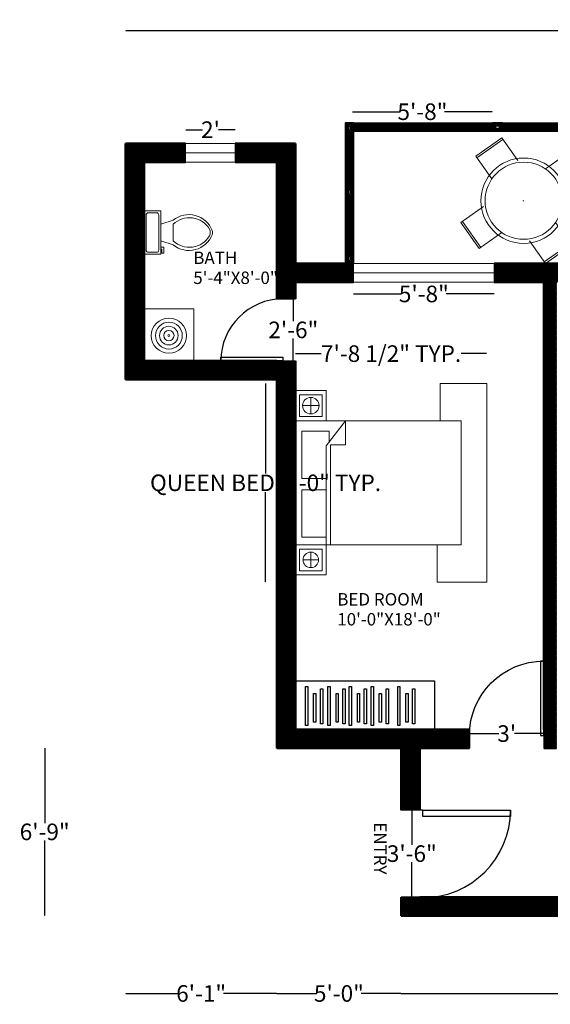
# Model space of a CAD drawing. Units: inches. Extents: x 348 to 1197, y 2602 to 3078.
# Tile 1 of 4: x 348 to 604, y 2602 to 3078. Entities that reach past the tile are written whole.
import ezdxf

# ---------------------------------------------------------------- set-up
doc = ezdxf.new("R2010")
doc.units = ezdxf.units.IN
doc.header["$MEASUREMENT"] = 0
for name, color, linetype, lineweight in [('A-ANNO-DIMS', 20, 'Continuous', 18), ('A-AREA-IDEN', 104, 'Continuous', 18), ('A-FLOR-CASE', 5, 'Continuous', 25), ('A-FLOR-FIXT', 9, 'Continuous', 18), ('A-WALL-PATT', 250, 'Continuous', 13), ('balcony', 201, 'Continuous', 25), ('bed', 5, 'Continuous', 18), ('doors', 1, 'Continuous', 25), ('table', 6, 'Continuous', 18), ('walls', 4, 'Continuous', 50), ('windows', 2, 'Continuous', 18)]:
    doc.layers.add(name, color=color, linetype=linetype, lineweight=lineweight)
doc.styles.get("Standard").update_dxf_attribs({"font": 'arial.ttf'})
doc.dimstyles.get("Standard").update_dxf_attribs({"dimtxt": 8, "dimasz": 0.18, "dimexe": 0.18, "dimexo": 0.0625, "dimgap": 0.09, "dimtad": 0, "dimtih": 1, "dimtoh": 1, "dimdec": 0, "dimzin": 0, "dimdsep": 46, "dimlunit": 3, "dimtxsty": 'Standard', "dimblk": 'DOT', "dimcen": 0.09, "dimse1": 1, "dimse2": 1, "dimadec": 0, "dimazin": 0, "dimtfac": 1, "dimtdec": 0, "dimtofl": 0, "dimtmove": 0, "dimatfit": 3, "dimfxl": 1, "dimtolj": 1, "dimtzin": 0, "dimarcsym": 0})

# ---------------------------------------------------------------- blocks, each defined once
blk = doc.blocks.new('*U8')
for p, q in [((0, 0), (0, -6)), ((24, 0), (24, -6))]:
    blk.add_line(p, q)
blk.add_lwpolyline([(0, 0), (0, 24), (1.75, 24), (1.75, 0)], close=True)
blk.add_arc((0, 0), 24, 360, 90)
blk = doc.blocks.new('*U10')
for p, q in [((0, 0), (0, -6)), ((30, 0), (30, -6))]:
    blk.add_line(p, q)
blk.add_lwpolyline([(0, 0), (0, 30), (1.75, 30), (1.75, 0)], close=True)
blk.add_arc((0, 0), 30, 0, 90)
blk = doc.blocks.new('*U9')
for p, q in [((0, 0), (0, -6)), ((36, 0), (36, -6))]:
    blk.add_line(p, q)
blk.add_lwpolyline([(0, 0), (0, 36), (1.75, 36), (1.75, 0)], close=True)
blk.add_arc((0, 0), 36, 0, 90)
blk = doc.blocks.new('*U13')
for p, q in [((5.98, 9.51), (1.98, 9.5)), ((7.99, 4.02), (13.99, 6.03)), ((13.99, 4.03), (14.01, -3.97)), ((8.01, -3.98), (14.01, -5.97)), ((8.01, -6.98), (9.51, -6.98)), ((8.52, -7.98), (8.02, -7.98)), ((8.52, -9.98), (8.52, -7.98)), ((9.51, -6.98), (9.52, -9.98)), ((9.52, -9.98), (8.52, -9.98))]:
    blk.add_line(p, q)
blk.add_lwpolyline([(7.98, 10.51), (-0.02, 10.5), (0.02, -10.5), (8.02, -10.48)], close=True)
for points in [[(0.98, 8.5), (1.02, -8.5)], [(7.02, -8.49), (6.98, 8.51)], [(2.02, -9.5), (6.02, -9.49)]]:
    blk.add_lwpolyline(points)
for centre, radius, start, end in [((6.11, 8.64), 0.884, 351.9774, 98.2376), ((1.86, 8.63), 0.884, 81.9774, 188.2376), ((21.59, -3.48), 12.17, 22.136, 128.6382), ((21.83, -4.16), 11.33, 31.1605, 133.7396), ((27.88, 0.05), 4, 335.8394, 24.3757), ((29, 0.05), 4, 344.9681, 15.247), ((21.57, 3.56), 12.17, 231.5766, 338.079), ((21.81, 4.24), 11.33, 226.4753, 329.0544), ((1.89, -8.62), 0.884, 171.9774, 278.2376), ((6.14, -8.61), 0.884, 261.9774, 8.2376)]:
    blk.add_arc(centre, radius, start, end)
blk = doc.blocks.new('*U14')
at = {"layer": 'table'}
for p, q in [((-7.7, -6.73), (-7.7, 6.73)), ((-7.7, 6.73), (7.7, 6.73)), ((-7.7, 5.73), (7.7, 5.73)), ((7.7, 6.73), (7.7, -6.73))]:
    blk.add_line(p, q, dxfattribs=at)
blk = doc.blocks.new('*U15')
at = {"layer": 'table', "transparency": 16777216}
blk.add_blockref('*U14', (596.31, 3015.18), dxfattribs=at)
for p, rotation in [((570.95, 2992.17), 90), ((619.32, 2989.82), 270), ((593.96, 2966.81), 180)]:
    blk.add_blockref('*U14', p, dxfattribs=dict(at, rotation=rotation))
blk = doc.blocks.new('_Dot')
at = {"color": 0, "linetype": 'ByBlock', "lineweight": -2}
blk.add_line((-0.5, 0), (-1, 0), dxfattribs=at)
at = {"color": 0, "linetype": 'ByBlock', "const_width": 0.5}
blk.add_lwpolyline([(-0.25, 0, 1), (0.25, 0, 1)], format="xyb", close=True, dxfattribs=at)
blk = doc.blocks.new('*D19')
at = {"layer": 'A-ANNO-DIMS', "color": 0, "lineweight": -2, "transparency": 16777216}
for p, q in [((428.5, 3024.92), (436.48, 3024.92)), ((452.14, 3024.92), (444.16, 3024.92))]:
    blk.add_line(p, q, dxfattribs=at)
at = {"layer": 'Defpoints', "color": 0, "transparency": 16777216}
for p in [(452.32, 3024.92), (428.32, 3018.2), (452.32, 3018.2)]:
    blk.add_point(p, dxfattribs=at)
at = {"layer": 'A-ANNO-DIMS', "color": 0, "lineweight": -2, "transparency": 16777216, "xscale": 0.18, "yscale": 0.18, "zscale": 0.18, "rotation": 180}
blk.add_blockref('_Dot', (428.32, 3024.92), dxfattribs=at)
at = {"layer": 'A-ANNO-DIMS', "color": 0, "lineweight": -2, "transparency": 16777216, "xscale": 0.18, "yscale": 0.18, "zscale": 0.18}
blk.add_blockref('_Dot', (452.32, 3024.92), dxfattribs=at)
at = {"layer": 'A-ANNO-DIMS', "color": 0, "transparency": 16777216, "insert": (440.32, 3024.92), "char_height": 8, "attachment_point": 5}
blk.add_mtext("\\A1;2'", dxfattribs=at)
blk = doc.blocks.new('*D20')
at = {"layer": 'A-ANNO-DIMS', "color": 0, "lineweight": -2, "transparency": 16777216}
for p, q in [((509, 3033.6), (531.92, 3033.6)), ((576.28, 3033.6), (553.36, 3033.6))]:
    blk.add_line(p, q, dxfattribs=at)
at = {"layer": 'Defpoints', "color": 0, "transparency": 16777216}
for p in [(576.46, 3033.6), (508.82, 3027.67), (576.46, 3027.67)]:
    blk.add_point(p, dxfattribs=at)
at = {"layer": 'A-ANNO-DIMS', "color": 0, "lineweight": -2, "transparency": 16777216, "xscale": 0.18, "yscale": 0.18, "zscale": 0.18, "rotation": 180}
blk.add_blockref('_Dot', (508.82, 3033.6), dxfattribs=at)
at = {"layer": 'A-ANNO-DIMS', "color": 0, "lineweight": -2, "transparency": 16777216, "xscale": 0.18, "yscale": 0.18, "zscale": 0.18}
blk.add_blockref('_Dot', (576.46, 3033.6), dxfattribs=at)
at = {"layer": 'A-ANNO-DIMS', "color": 0, "transparency": 16777216, "insert": (542.64, 3033.6), "char_height": 8, "attachment_point": 5}
blk.add_mtext('\\A1;5\'-8"', dxfattribs=at)
blk = doc.blocks.new('*D23')
at = {"layer": 'A-ANNO-DIMS', "color": 0, "lineweight": -2, "transparency": 16777216}
for p, q in [((537.51, 2696.02), (537.51, 2679.38)), ((537.51, 2654.38), (537.51, 2671.03))]:
    blk.add_line(p, q, dxfattribs=at)
at = {"layer": 'Defpoints', "color": 0, "transparency": 16777216}
for p in [(532.32, 2696.2), (532.32, 2654.2), (537.51, 2654.2)]:
    blk.add_point(p, dxfattribs=at)
at = {"layer": 'A-ANNO-DIMS', "color": 0, "lineweight": -2, "transparency": 16777216, "xscale": 0.18, "yscale": 0.18, "zscale": 0.18}
for p, rotation in [((537.51, 2696.2), 90), ((537.51, 2654.2), 270)]:
    blk.add_blockref('_Dot', p, dxfattribs=dict(at, rotation=rotation))
at = {"layer": 'A-ANNO-DIMS', "color": 0, "transparency": 16777216, "insert": (537.51, 2675.2), "char_height": 8, "attachment_point": 5}
blk.add_mtext('\\A1;3\'-6"', dxfattribs=at)
blk = doc.blocks.new('*D24')
at = {"layer": 'A-ANNO-DIMS', "color": 0, "lineweight": -2, "transparency": 16777216}
for p, q in [((565.5, 2733.19), (579.55, 2733.19)), ((601.14, 2733.19), (587.09, 2733.19))]:
    blk.add_line(p, q, dxfattribs=at)
at = {"layer": 'Defpoints', "color": 0, "transparency": 16777216}
for p in [(601.32, 2733.19), (565.32, 2726.2), (601.32, 2726.2)]:
    blk.add_point(p, dxfattribs=at)
at = {"layer": 'A-ANNO-DIMS', "color": 0, "lineweight": -2, "transparency": 16777216, "xscale": 0.18, "yscale": 0.18, "zscale": 0.18, "rotation": 180}
blk.add_blockref('_Dot', (565.32, 2733.19), dxfattribs=at)
at = {"layer": 'A-ANNO-DIMS', "color": 0, "lineweight": -2, "transparency": 16777216, "xscale": 0.18, "yscale": 0.18, "zscale": 0.18}
blk.add_blockref('_Dot', (601.32, 2733.19), dxfattribs=at)
at = {"layer": 'A-ANNO-DIMS', "color": 0, "transparency": 16777216, "insert": (583.32, 2733.19), "char_height": 8, "attachment_point": 5}
blk.add_mtext("\\A1;3'", dxfattribs=at)
blk = doc.blocks.new('*D28')
at = {"layer": 'A-ANNO-DIMS', "color": 0, "lineweight": -2, "transparency": 16777216}
for p, q in [((509.5, 2945.57), (532.59, 2945.57)), ((577.14, 2945.57), (554.04, 2945.57))]:
    blk.add_line(p, q, dxfattribs=at)
at = {"layer": 'Defpoints', "color": 0, "transparency": 16777216}
for p in [(509.32, 2951.2), (577.32, 2951.2), (577.32, 2945.57)]:
    blk.add_point(p, dxfattribs=at)
at = {"layer": 'A-ANNO-DIMS', "color": 0, "lineweight": -2, "transparency": 16777216, "xscale": 0.18, "yscale": 0.18, "zscale": 0.18, "rotation": 180}
blk.add_blockref('_Dot', (509.32, 2945.57), dxfattribs=at)
at = {"layer": 'A-ANNO-DIMS', "color": 0, "lineweight": -2, "transparency": 16777216, "xscale": 0.18, "yscale": 0.18, "zscale": 0.18}
blk.add_blockref('_Dot', (577.32, 2945.57), dxfattribs=at)
at = {"layer": 'A-ANNO-DIMS', "color": 0, "transparency": 16777216, "insert": (543.32, 2945.57), "char_height": 8, "attachment_point": 5}
blk.add_mtext('\\A1;5\'-8"', dxfattribs=at)
blk = doc.blocks.new('*D29')
at = {"layer": 'A-ANNO-DIMS', "color": 0, "lineweight": -2, "transparency": 16777216}
for p, q in [((480.31, 2943.02), (480.31, 2932.38)), ((480.31, 2913.38), (480.31, 2924.03))]:
    blk.add_line(p, q, dxfattribs=at)
at = {"layer": 'Defpoints', "color": 0, "transparency": 16777216}
for p in [(480.31, 2943.2), (481.32, 2943.2), (481.32, 2913.2)]:
    blk.add_point(p, dxfattribs=at)
at = {"layer": 'A-ANNO-DIMS', "color": 0, "lineweight": -2, "transparency": 16777216, "xscale": 0.18, "yscale": 0.18, "zscale": 0.18}
for p, rotation in [((480.31, 2943.2), 90), ((480.31, 2913.2), 270)]:
    blk.add_blockref('_Dot', p, dxfattribs=dict(at, rotation=rotation))
at = {"layer": 'A-ANNO-DIMS', "color": 0, "transparency": 16777216, "insert": (480.31, 2928.2), "char_height": 8, "attachment_point": 5}
blk.add_mtext('\\A1;2\'-6"', dxfattribs=at)
blk = doc.blocks.new('BED-QUEEN')
for p, q in [((24, 96), (0, 96)), ((0, 96), (0, 0)), ((24, 78), (24, 96)), ((92.39, 78), (12.39, 78)), ((12.39, 78), (12.39, 18)), ((75.49, 78), (75.49, 29.69)), ((77.49, 78), (77.49, 30.16)), ((77.49, 30.16), (68.23, 18)), ((68.23, 29.62), (75.49, 29.69)), ((68.23, 18), (68.23, 29.62)), ((12.39, 18), (92.39, 18)), ((22.56, 18), (22.56, 0)), ((22.56, 0), (0, 0))]:
    blk.add_line(p, q)
for points in [[(77.49, 51.42), (89.26, 51.42), (89.26, 74.34), (77.49, 74.34)], [(76.09, 28.32), (76.09, 23.06), (89.26, 23.06), (89.26, 45.98), (77.49, 45.98)]]:
    blk.add_lwpolyline(points)
blk = doc.blocks.new('WARDROBE-HANGER-SET')
for points in [[(0, 18.89), (1.11, 18.89), (1.11, 0), (0, 0)], [(3.89, 15.56), (5.01, 15.56), (5.01, 1.67), (3.89, 1.67)], [(7.23, 17.78), (8.34, 17.78), (8.34, 0.83), (7.23, 0.83)], [(10.85, 18.89), (11.96, 18.89), (11.96, 0), (10.85, 0)], [(14.74, 15.56), (15.86, 15.56), (15.86, 1.67), (14.74, 1.67)], [(18.08, 17.78), (19.19, 17.78), (19.19, 0.83), (18.08, 0.83)], [(21.14, 18.89), (22.25, 18.89), (22.25, 0), (21.14, 0)], [(25.04, 15.56), (26.15, 15.56), (26.15, 1.67), (25.04, 1.67)], [(28.37, 17.78), (29.49, 17.78), (29.49, 0.83), (28.37, 0.83)], [(31.71, 18.89), (32.82, 18.89), (32.82, 0), (31.71, 0)], [(35.61, 15.56), (36.72, 15.56), (36.72, 1.67), (35.61, 1.67)], [(38.94, 17.78), (40.06, 17.78), (40.06, 0.83), (38.94, 0.83)], [(44.51, 18.89), (45.62, 18.89), (45.62, 0), (44.51, 0)], [(48.4, 15.56), (49.51, 15.56), (49.51, 1.67), (48.4, 1.67)], [(51.74, 17.78), (52.85, 17.78), (52.85, 0.83), (51.74, 0.83)]]:
    blk.add_lwpolyline(points, close=True)
blk = doc.blocks.new('RAIL-POST-CORE')
for points in [[(0, 0), (3, 0), (3, 3.9), (0, 3.9)], [(0.5, 0.5), (2.5, 0.5), (2.5, 3.4), (0.5, 3.4)], [(1, 1), (2, 1), (2, 2.9), (1, 2.9)]]:
    blk.add_lwpolyline(points, close=True)
blk = doc.blocks.new('BALCONY-TABLE-ROUND')
for radius in [20.64, 18.64]:
    blk.add_circle((20.64, 20.64), radius)
blk = doc.blocks.new('BASIN-ROUND')
for radius in [8.49, 8.49, 8.49, 6.49, 4.49, 4.49, 2.49, 0.487]:
    blk.add_circle((8.49, 8.49), radius)
blk = doc.blocks.new('*D54')
at = {"layer": 'A-ANNO-DIMS', "color": 0, "lineweight": -2, "transparency": 16777216}
for p, q in [((466.91, 2902.16), (466.91, 2858.82)), ((466.91, 2806.52), (466.91, 2849.87))]:
    blk.add_line(p, q, dxfattribs=at)
at = {"layer": 'Defpoints', "color": 0, "transparency": 16777216}
for p in [(481.31, 2902.34), (466.91, 2806.34), (481.31, 2806.34)]:
    blk.add_point(p, dxfattribs=at)
at = {"layer": 'A-ANNO-DIMS', "color": 0, "lineweight": -2, "transparency": 16777216, "xscale": 0.18, "yscale": 0.18, "zscale": 0.18}
for p, rotation in [((466.91, 2902.34), 90), ((466.91, 2806.34), 270)]:
    blk.add_blockref('_Dot', p, dxfattribs=dict(at, rotation=rotation))
at = {"layer": 'A-ANNO-DIMS', "color": 0, "transparency": 16777216, "insert": (466.91, 2854.34), "char_height": 8, "attachment_point": 5}
blk.add_mtext('\\A1;QUEEN BED 8\'-0" TYP.', dxfattribs=at)
blk = doc.blocks.new('*D55')
at = {"layer": 'A-ANNO-DIMS', "color": 0, "lineweight": -2, "transparency": 16777216}
for p, q in [((481.49, 2916.74), (493.75, 2916.74)), ((573.52, 2916.74), (561.27, 2916.74))]:
    blk.add_line(p, q, dxfattribs=at)
at = {"layer": 'Defpoints', "color": 0, "transparency": 16777216}
for p in [(481.31, 2916.74), (481.31, 2902.34), (573.7, 2902.34)]:
    blk.add_point(p, dxfattribs=at)
at = {"layer": 'A-ANNO-DIMS', "color": 0, "lineweight": -2, "transparency": 16777216, "xscale": 0.18, "yscale": 0.18, "zscale": 0.18, "rotation": 180}
blk.add_blockref('_Dot', (481.31, 2916.74), dxfattribs=at)
at = {"layer": 'A-ANNO-DIMS', "color": 0, "lineweight": -2, "transparency": 16777216, "xscale": 0.18, "yscale": 0.18, "zscale": 0.18}
blk.add_blockref('_Dot', (573.7, 2916.74), dxfattribs=at)
at = {"layer": 'A-ANNO-DIMS', "color": 0, "transparency": 16777216, "insert": (527.51, 2916.74), "char_height": 8, "attachment_point": 5}
blk.add_mtext('\\A1;7\'-8 1/2" TYP.', dxfattribs=at)
blk = doc.blocks.new('*D68')
at = {"layer": 'A-ANNO-DIMS', "color": 0, "lineweight": -2, "transparency": 16777216}
for p, q in [((399.5, 3072.8), (739.99, 3072.8)), ((1108.14, 3072.8), (767.65, 3072.8))]:
    blk.add_line(p, q, dxfattribs=at)
at = {"layer": 'Defpoints', "color": 0, "transparency": 16777216}
for p in [(1108.32, 3072.8), (1108.32, 3028.2), (399.32, 3018.2)]:
    blk.add_point(p, dxfattribs=at)
at = {"layer": 'A-ANNO-DIMS', "color": 0, "lineweight": -2, "transparency": 16777216, "xscale": 0.18, "yscale": 0.18, "zscale": 0.18, "rotation": 180}
blk.add_blockref('_Dot', (399.32, 3072.8), dxfattribs=at)
at = {"layer": 'A-ANNO-DIMS', "color": 0, "lineweight": -2, "transparency": 16777216, "xscale": 0.18, "yscale": 0.18, "zscale": 0.18}
blk.add_blockref('_Dot', (1108.32, 3072.8), dxfattribs=at)
at = {"layer": 'A-ANNO-DIMS', "color": 0, "transparency": 16777216, "insert": (753.82, 3072.8), "char_height": 8, "attachment_point": 5}
blk.add_mtext('\\A1;59\'-1"', dxfattribs=at)
blk = doc.blocks.new('*D70')
at = {"layer": 'A-ANNO-DIMS', "color": 0, "lineweight": -2, "transparency": 16777216}
for p, q in [((399.5, 2607.65), (425.07, 2607.65)), ((472.14, 2607.65), (446.56, 2607.65))]:
    blk.add_line(p, q, dxfattribs=at)
at = {"layer": 'Defpoints', "color": 0, "transparency": 16777216}
for p in [(399.32, 2904.2), (472.32, 2904.2), (472.32, 2607.65)]:
    blk.add_point(p, dxfattribs=at)
at = {"layer": 'A-ANNO-DIMS', "color": 0, "lineweight": -2, "transparency": 16777216, "xscale": 0.18, "yscale": 0.18, "zscale": 0.18, "rotation": 180}
blk.add_blockref('_Dot', (399.32, 2607.65), dxfattribs=at)
at = {"layer": 'A-ANNO-DIMS', "color": 0, "lineweight": -2, "transparency": 16777216, "xscale": 0.18, "yscale": 0.18, "zscale": 0.18}
blk.add_blockref('_Dot', (472.32, 2607.65), dxfattribs=at)
at = {"layer": 'A-ANNO-DIMS', "color": 0, "transparency": 16777216, "insert": (435.82, 2607.65), "char_height": 8, "attachment_point": 5}
blk.add_mtext('\\A1;6\'-1"', dxfattribs=at)
blk = doc.blocks.new('*D71')
at = {"layer": 'A-ANNO-DIMS', "color": 0, "lineweight": -2, "transparency": 16777216}
for p, q in [((472.5, 2607.65), (491.59, 2607.65)), ((532.14, 2607.65), (513.04, 2607.65))]:
    blk.add_line(p, q, dxfattribs=at)
at = {"layer": 'Defpoints', "color": 0, "transparency": 16777216}
for p in [(472.32, 2726.2), (532.32, 2726.2), (532.32, 2607.65)]:
    blk.add_point(p, dxfattribs=at)
at = {"layer": 'A-ANNO-DIMS', "color": 0, "lineweight": -2, "transparency": 16777216, "xscale": 0.18, "yscale": 0.18, "zscale": 0.18, "rotation": 180}
blk.add_blockref('_Dot', (472.32, 2607.65), dxfattribs=at)
at = {"layer": 'A-ANNO-DIMS', "color": 0, "lineweight": -2, "transparency": 16777216, "xscale": 0.18, "yscale": 0.18, "zscale": 0.18}
blk.add_blockref('_Dot', (532.32, 2607.65), dxfattribs=at)
at = {"layer": 'A-ANNO-DIMS', "color": 0, "transparency": 16777216, "insert": (502.32, 2607.65), "char_height": 8, "attachment_point": 5}
blk.add_mtext('\\A1;5\'-0"', dxfattribs=at)
blk = doc.blocks.new('*D72')
at = {"layer": 'A-ANNO-DIMS', "color": 0, "lineweight": -2, "transparency": 16777216}
for p, q in [((532.5, 2607.65), (678.92, 2607.65)), ((853.14, 2607.65), (706.72, 2607.65))]:
    blk.add_line(p, q, dxfattribs=at)
at = {"layer": 'Defpoints', "color": 0, "transparency": 16777216}
for p in [(532.32, 2645.2), (853.32, 2645.2), (853.32, 2607.65)]:
    blk.add_point(p, dxfattribs=at)
at = {"layer": 'A-ANNO-DIMS', "color": 0, "lineweight": -2, "transparency": 16777216, "xscale": 0.18, "yscale": 0.18, "zscale": 0.18, "rotation": 180}
blk.add_blockref('_Dot', (532.32, 2607.65), dxfattribs=at)
at = {"layer": 'A-ANNO-DIMS', "color": 0, "lineweight": -2, "transparency": 16777216, "xscale": 0.18, "yscale": 0.18, "zscale": 0.18}
blk.add_blockref('_Dot', (853.32, 2607.65), dxfattribs=at)
at = {"layer": 'A-ANNO-DIMS', "color": 0, "transparency": 16777216, "insert": (692.82, 2607.65), "char_height": 8, "attachment_point": 5}
blk.add_mtext('\\A1;26\'-9"', dxfattribs=at)
blk = doc.blocks.new('*D75')
at = {"layer": 'A-ANNO-DIMS', "color": 0, "lineweight": -2, "transparency": 16777216}
for p, q in [((360.29, 2726.02), (360.29, 2689.88)), ((360.29, 2645.38), (360.29, 2681.53))]:
    blk.add_line(p, q, dxfattribs=at)
at = {"layer": 'Defpoints', "color": 0, "transparency": 16777216}
for p in [(472.32, 2726.2), (360.29, 2645.2), (532.32, 2645.2)]:
    blk.add_point(p, dxfattribs=at)
at = {"layer": 'A-ANNO-DIMS', "color": 0, "lineweight": -2, "transparency": 16777216, "xscale": 0.18, "yscale": 0.18, "zscale": 0.18}
for p, rotation in [((360.29, 2726.2), 90), ((360.29, 2645.2), 270)]:
    blk.add_blockref('_Dot', p, dxfattribs=dict(at, rotation=rotation))
at = {"layer": 'A-ANNO-DIMS', "color": 0, "transparency": 16777216, "insert": (360.29, 2685.7), "char_height": 8, "attachment_point": 5}
blk.add_mtext('\\A1;6\'-9"', dxfattribs=at)
blk = doc.blocks.new('*D82')
at = {"layer": 'A-ANNO-DIMS', "color": 0, "lineweight": -2, "transparency": 16777216}
for p, q in [((591.41, 2990.59), (591.59, 2990.59)), ((591.5, 2990.5), (591.5, 2990.68)), ((621.33, 2990.59), (610.32, 2990.59))]:
    blk.add_line(p, q, dxfattribs=at)
at = {"layer": 'Defpoints', "color": 0, "transparency": 16777216}
for p in [(572.87, 2990.6), (610.14, 2990.59)]:
    blk.add_point(p, dxfattribs=at)
at = {"layer": 'A-ANNO-DIMS', "color": 0, "lineweight": -2, "transparency": 16777216, "xscale": 0.18, "yscale": 0.18, "zscale": 0.18, "rotation": 179.9894899347775}
blk.add_blockref('_Dot', (610.14, 2990.59), dxfattribs=at)
at = {"layer": 'A-ANNO-DIMS', "color": 0, "transparency": 16777216, "insert": (654.17, 2990.59), "char_height": 8, "attachment_point": 5}
blk.add_mtext('\\A1;2X ∅3\'-1 1/2"', dxfattribs=at)

msp = doc.modelspace()

# ---------------------------------------------------------------- hatches: boundary and pattern name
at = {"layer": 'A-WALL-PATT'}
h = msp.add_hatch(dxfattribs=at)
h.set_pattern_fill('ANSI31', color=256, scale=1.5)
h.paths.add_polyline_path([(481.32, 2951.2), (509.32, 2951.2), (509.32, 2960.2), (505.32, 2960.2), (481.32, 2960.2), (481.32, 3018.2), (452.32, 3018.2), (452.32, 3009.2), (472.32, 3009.2), (472.32, 2943.2), (481.32, 2943.2)], flags=17)
h.paths.add_polyline_path([(428.32, 3018.2), (399.32, 3018.2), (399.32, 2904.2), (472.32, 2904.2), (472.32, 2726.2), (532.32, 2726.2), (532.32, 2696.2), (541.32, 2696.2), (541.32, 2726.2), (565.32, 2726.2), (565.32, 2735.2), (481.32, 2735.2), (481.32, 2758.72), (481.32, 2809.83), (481.31, 2809.83), (481.31, 2824.34), (481.31, 2884.34), (481.31, 2884.34), (481.31, 2898.86), (481.32, 2913.2), (472.32, 2913.2), (408.32, 2913.2), (408.32, 3009.2), (428.32, 3009.2)])
h.paths.add_polyline_path([(796.32, 2654.2), (769.32, 2654.2), (769.32, 2753.2), (769.32, 2759.2), (763.32, 2759.2), (763.32, 2735.2), (763.32, 2654.2), (541.32, 2654.2), (532.32, 2654.2), (532.32, 2645.2), (796.32, 2645.2)])
h.paths.add_polyline_path([(853.32, 2726.2), (1018.32, 2726.2), (1018.32, 2703.7), (1027.32, 2703.7), (1027.32, 2729.2), (1057.32, 2729.2), (1057.32, 2735.2), (919.32, 2735.2), (919.32, 2758.72), (919.32, 2765.2), (913.32, 2765.2), (913.32, 2735.2), (853.32, 2735.2), (853.32, 2759.2), (799.32, 2759.2), (799.32, 2753.2), (847.32, 2753.2), (847.32, 2654.2), (820.32, 2654.2), (820.32, 2645.2), (853.32, 2645.2)])
h.paths.add_polyline_path([(640.32, 2960.2), (577.32, 2960.2), (577.32, 2951.2), (601.32, 2951.2), (601.32, 2735.2), (601.32, 2726.2), (607.32, 2726.2), (607.32, 2951.2), (640.32, 2951.2)])
h.paths.add_polyline_path([(877.32, 2960.2), (688.32, 2960.2), (688.32, 2951.2), (745.32, 2951.2), (745.32, 2837.2), (751.32, 2837.2), (751.32, 2951.2), (847.32, 2951.2), (847.32, 2807.2), (751.32, 2807.2), (745.32, 2807.2), (745.32, 2801.2), (853.32, 2801.2), (853.32, 2807.2), (853.32, 2951.2), (877.32, 2951.2)])
h.paths.add_polyline_path([(1003.32, 2960.2), (949.32, 2960.2), (949.32, 2951.2), (973.32, 2951.2), (973.32, 2807.2), (906.15, 2807.2), (893.32, 2807.2), (893.32, 2801.2), (913.32, 2801.2), (919.32, 2801.2), (955.32, 2801.2), (979.32, 2801.2), (979.32, 2951.2), (1003.32, 2951.2)])
h.paths.add_polyline_path([(1108.32, 2960.2), (1104.32, 2960.2), (1075.32, 2960.2), (1075.32, 2951.2), (1099.32, 2951.2), (1099.32, 2735.2), (1087.32, 2735.2), (1087.32, 2729.2), (1099.32, 2729.2), (1099.32, 2654.2), (1027.32, 2654.2), (1027.32, 2679.7), (1018.32, 2679.7), (1018.32, 2645.2), (1108.32, 2645.2)])
h.paths.add_polyline_path([(509.32, 2992.2), (505.32, 2992.2), (505.32, 2965.1), (509.32, 2965.1)], flags=16)
h.paths.add_polyline_path([(509.32, 3023.27), (505.32, 3023.27), (505.32, 2997.1), (509.32, 2997.1)])
h.paths.add_polyline_path([(576.46, 3028.2), (509.32, 3028.2), (509.32, 3024.2), (576.46, 3024.2)])
h.paths.add_polyline_path([(624.46, 3028.2), (581.36, 3028.2), (581.36, 3024.2), (624.46, 3024.2)])
h.paths.add_polyline_path([(672.46, 3028.2), (629.36, 3028.2), (629.36, 3024.2), (672.46, 3024.2)])
h.paths.add_polyline_path([(720.46, 3028.2), (677.36, 3028.2), (677.36, 3024.2), (720.46, 3024.2)])
h.paths.add_polyline_path([(768.46, 3028.2), (725.36, 3028.2), (725.36, 3024.2), (768.46, 3024.2)])
h.paths.add_polyline_path([(804.46, 3028.2), (773.36, 3028.2), (773.36, 3024.2), (804.46, 3024.2)])
h.paths.add_polyline_path([(852.46, 3028.2), (809.36, 3028.2), (809.36, 3024.2), (852.46, 3024.2)])
h.paths.add_polyline_path([(900.46, 3028.2), (857.36, 3028.2), (857.36, 3024.2), (900.46, 3024.2)])
h.paths.add_polyline_path([(948.46, 3028.2), (905.36, 3028.2), (905.36, 3024.2), (948.46, 3024.2)])
h.paths.add_polyline_path([(996.46, 3028.2), (953.36, 3028.2), (953.36, 3024.2), (996.46, 3024.2)])
h.paths.add_polyline_path([(1056.46, 3028.2), (1001.36, 3028.2), (1001.36, 3024.2), (1056.46, 3024.2)])
h.paths.add_polyline_path([(1103.42, 3028.2), (1061.36, 3028.2), (1061.36, 3024.2), (1103.42, 3024.2)])
h.paths.add_polyline_path([(1108.32, 3024.17), (1104.32, 3024.17), (1104.32, 2994.89), (1108.32, 2994.89)])
h.paths.add_polyline_path([(1108.32, 2989.99), (1104.32, 2989.99), (1104.32, 2965.1), (1108.32, 2965.1)])

# ---------------------------------------------------------------- linework, layer by layer
at = {"layer": 'A-FLOR-CASE'}
msp.add_lwpolyline([(481.32, 2758.72), (548.49, 2758.72), (548.49, 2735.2), (481.32, 2735.2)], close=True, dxfattribs=at)
at = {"layer": 'A-FLOR-FIXT'}
for p, q in [((408.32, 2938.33), (432.32, 2938.33)), ((432.32, 2938.33), (432.32, 2913.2))]:
    msp.add_line(p, q, dxfattribs=at)
at = {"layer": 'balcony'}
for p, q in [((505.32, 3028.2), (505.32, 2960.2)), ((505.32, 3028.2), (1108.32, 3028.2)), ((509.32, 3024.2), (1104.32, 3024.2)), ((509.32, 3024.2), (509.32, 2960.2))]:
    msp.add_line(p, q, dxfattribs=at)
for points in [[(505.32, 3023.27), (509.32, 3023.27), (509.32, 3028.17), (505.32, 3028.17)], [(505.82, 3023.77), (508.82, 3023.77), (508.82, 3027.67), (505.82, 3027.67)], [(506.32, 3024.27), (508.32, 3024.27), (508.32, 3027.17), (506.32, 3027.17)], [(506.82, 3024.77), (507.82, 3024.77), (507.82, 3026.67), (506.82, 3026.67)], [(581.36, 3024.17), (581.36, 3028.17), (576.46, 3028.17), (576.46, 3024.17)], [(505.32, 2992.2), (509.32, 2992.2), (509.32, 2997.1), (505.32, 2997.1)], [(505.32, 2960.2), (509.32, 2960.2), (509.32, 2965.1), (505.32, 2965.1)], [(505.82, 2960.7), (508.82, 2960.7), (508.82, 2964.6), (505.82, 2964.6)]]:
    msp.add_lwpolyline(points, close=True, dxfattribs=at)
at = {"layer": 'bed'}
for p, q in [((488.76, 2887.61), (488.76, 2895.59)), ((484.77, 2891.6), (492.75, 2891.6)), ((488.76, 2813.34), (488.76, 2820.84)), ((492.51, 2817.09), (485.01, 2817.09))]:
    msp.add_line(p, q, dxfattribs=at)
for points in [[(481.31, 2898.86), (496.21, 2898.86), (496.21, 2884.34), (481.31, 2884.34)], [(483.31, 2896.86), (494.21, 2896.86), (494.21, 2886.34), (483.31, 2886.34)], [(481.31, 2824.34), (496.21, 2824.34), (496.21, 2809.83), (481.31, 2809.83)], [(483.31, 2822.34), (494.21, 2822.34), (494.21, 2811.83), (483.31, 2811.83)]]:
    msp.add_lwpolyline(points, close=True, dxfattribs=at)
for centre, radius in [((488.76, 2891.6), 3.99), ((488.76, 2817.09), 3.75)]:
    msp.add_circle(centre, radius, dxfattribs=at)
at = {"layer": 'doors'}
for p, q in [((472.32, 2943.2), (481.32, 2943.2)), ((472.32, 2913.2), (481.32, 2913.2)), ((565.32, 2735.2), (565.32, 2726.2)), ((601.32, 2735.2), (601.32, 2726.2)), ((541.32, 2696.2), (532.32, 2696.2)), ((541.32, 2654.2), (532.32, 2654.2))]:
    msp.add_line(p, q, dxfattribs=at)
at = {"layer": 'walls'}
for p, q in [((399.32, 3018.2), (399.32, 2904.2)), ((428.32, 3018.2), (399.32, 3018.2)), ((481.32, 3018.2), (452.32, 3018.2)), ((481.32, 3018.2), (481.32, 2960.2)), ((408.32, 3009.2), (408.32, 2913.2)), ((428.32, 3009.2), (408.32, 3009.2)), ((472.32, 3009.2), (452.32, 3009.2)), ((472.32, 3009.2), (472.32, 2943.2)), ((481.32, 2960.2), (509.32, 2960.2)), ((577.32, 2960.2), (640.32, 2960.2)), ((481.32, 2951.2), (509.32, 2951.2)), ((481.32, 2951.2), (481.32, 2943.2)), ((577.32, 2951.2), (601.32, 2951.2)), ((601.32, 2951.2), (601.32, 2735.2)), ((472.32, 2913.2), (408.32, 2913.2)), ((481.32, 2913.2), (481.32, 2735.2)), ((472.32, 2904.2), (399.32, 2904.2)), ((472.32, 2904.2), (472.32, 2726.2)), ((481.32, 2735.2), (565.32, 2735.2)), ((532.32, 2726.2), (472.32, 2726.2)), ((532.32, 2726.2), (532.32, 2696.2)), ((541.32, 2726.2), (541.32, 2696.2)), ((541.32, 2726.2), (565.32, 2726.2)), ((601.32, 2726.2), (607.32, 2726.2)), ((532.32, 2654.2), (532.32, 2645.2)), ((541.32, 2654.2), (763.32, 2654.2)), ((532.32, 2645.2), (796.32, 2645.2))]:
    msp.add_line(p, q, dxfattribs=at)
at = {"layer": 'windows'}
for p, q in [((428.32, 3009.2), (428.32, 3018.2)), ((428.32, 3018.2), (452.32, 3018.2)), ((452.32, 3009.2), (452.32, 3018.2)), ((428.32, 3013.7), (452.32, 3013.7)), ((428.32, 3009.2), (452.32, 3009.2)), ((509.32, 2951.2), (509.32, 2960.2)), ((509.32, 2960.2), (577.32, 2960.2)), ((577.32, 2951.2), (577.32, 2960.2)), ((509.32, 2955.7), (577.32, 2955.7)), ((577.32, 2951.2), (509.32, 2951.2))]:
    msp.add_line(p, q, dxfattribs=at)

# ---------------------------------------------------------------- block references
at = {"layer": 'A-FLOR-CASE'}
msp.add_blockref('WARDROBE-HANGER-SET', (486.18, 2737.05), dxfattribs=at)
at = {"layer": 'A-FLOR-FIXT'}
for name, p, rotation in [('*U13', (408.32, 2975.23), 359.8924611627634), ('BASIN-ROUND', (426.41, 2915.14), 75.96375653207353)]:
    msp.add_blockref(name, p, dxfattribs=dict(at, rotation=rotation))
at = {"layer": 'balcony', "rotation": 90.00000000001351}
msp.add_blockref('RAIL-POST-CORE', (580.86, 3024.67), dxfattribs=at)
at = {"layer": 'balcony'}
for p in [(505.82, 2992.7), (505.82, 2960.7)]:
    msp.add_blockref('RAIL-POST-CORE', p, dxfattribs=at)
at = {"layer": 'bed', "rotation": 180}
msp.add_blockref('BED-QUEEN', (573.7, 2902.34), dxfattribs=at)
at = {"layer": 'doors', "rotation": 90}
msp.add_blockref('*U10', (475.32, 2913.2), dxfattribs=at)
at = {"layer": 'doors', "xscale": -1}
msp.add_blockref('*U9', (601.32, 2732.2), dxfattribs=at)
at = {"layer": 'doors', "xscale": 1.760946222533251, "yscale": 1.760946222533251, "zscale": 1.760946222533251, "rotation": 270}
msp.add_blockref('*U8', (542.88, 2696.2), dxfattribs=at)
at = {"layer": 'table', "rotation": 215.168770522954}
msp.add_blockref('*U15', (-644.77, 5778.4), dxfattribs=at)
at = {"layer": 'table'}
msp.add_blockref('BALCONY-TABLE-ROUND', (570.87, 2969.95), dxfattribs=at)

# ---------------------------------------------------------------- texts
at = {"layer": 'A-AREA-IDEN'}
for s, p in [('BATH ', (432.02, 2960.02)), ('5\'-4"X8\'-0"', (432.02, 2950.38)), ('BED ROOM ', (501.54, 2795.05)), ('10\'-0"X18\'-0"', (501.54, 2785.41))]:
    msp.add_text(s, height=6, dxfattribs=at).set_placement(p)
msp.add_text('ENTRY ', height=6, rotation=270, dxfattribs=at).set_placement((519.3, 2690.31))

# ---------------------------------------------------------------- dimensions: what is measured, and where the dimension line sits
at = {"layer": 'A-ANNO-DIMS'}
for base, p1, p2, override, picture, middle in [((1108.32, 3072.8), (399.32, 3018.2), (1108.32, 3028.2), {"dimdec": 1, "dimlfac": 1, "dimrnd": 0, "dimzin": 1, "dimdsep": 46, "dimlunit": 4, "dimfrac": 2}, '*D68', (753.82, 3072.8)), ((576.46, 3033.6), (508.82, 3027.67), (576.46, 3027.67), {"dimclrd": 0, "dimclre": 0, "dimclrt": 0}, '*D20', (542.64, 3033.6)), ((452.32, 3024.92), (428.32, 3018.2), (452.32, 3018.2), {"dimclrd": 0, "dimclre": 0, "dimclrt": 0}, '*D19', (440.32, 3024.92)), ((577.32, 2945.57), (509.32, 2951.2), (577.32, 2951.2), {"dimclrd": 0, "dimclre": 0, "dimclrt": 0}, '*D28', (543.32, 2945.57)), ((472.32, 2607.65), (399.32, 2904.2), (472.32, 2904.2), {"dimdec": 1, "dimlfac": 1, "dimrnd": 0, "dimzin": 1, "dimdsep": 46, "dimlunit": 4, "dimfrac": 2}, '*D70', (435.82, 2607.65)), ((601.32, 2733.19), (565.32, 2726.2), (601.32, 2726.2), {"dimclrd": 0, "dimclre": 0, "dimclrt": 0}, '*D24', (583.32, 2733.19)), ((532.32, 2607.65), (472.32, 2726.2), (532.32, 2726.2), {"dimdec": 1, "dimlfac": 1, "dimrnd": 0, "dimzin": 1, "dimdsep": 46, "dimlunit": 4, "dimfrac": 2}, '*D71', (502.32, 2607.65)), ((853.32, 2607.65), (532.32, 2645.2), (853.32, 2645.2), {"dimdec": 1, "dimlfac": 1, "dimrnd": 0, "dimzin": 1, "dimdsep": 46, "dimlunit": 4, "dimfrac": 2}, '*D72', (692.82, 2607.65))]:
    dim = msp.add_linear_dim(base=base, p1=p1, p2=p2, dimstyle='Standard', override=override, dxfattribs=at)
    dim.commit()
    dim.dimension.update_dxf_attribs({"geometry": picture, "text_midpoint": middle})
dim = msp.add_diameter_dim_2p(p1=(572.87, 2990.6), p2=(610.14, 2990.59), text='2X <>', dimstyle='Standard', override={"dimdec": 1, "dimlfac": 1, "dimrnd": 0, "dimzin": 1, "dimdsep": 46, "dimlunit": 4, "dimfrac": 2}, dxfattribs=at)
dim.commit()
dim.dimension.update_dxf_attribs({"geometry": '*D82', "text_midpoint": (621.33, 2990.59), "dimtype": 163})
for base, p1, p2, override, picture, middle in [((480.31, 2943.2), (481.32, 2913.2), (481.32, 2943.2), {"dimclrd": 0, "dimclre": 0, "dimclrt": 0}, '*D29', (480.31, 2928.2)), ((360.29, 2645.2), (472.32, 2726.2), (532.32, 2645.2), {"dimdec": 1, "dimlfac": 1, "dimrnd": 0, "dimzin": 1, "dimdsep": 46, "dimlunit": 4, "dimfrac": 2}, '*D75', (360.29, 2685.7)), ((537.51, 2654.2), (532.32, 2696.2), (532.32, 2654.2), {"dimclrd": 0, "dimclre": 0, "dimclrt": 0}, '*D23', (537.51, 2675.2))]:
    dim = msp.add_linear_dim(base=base, p1=p1, p2=p2, angle=90, dimstyle='Standard', override=override, dxfattribs=at)
    dim.commit()
    dim.dimension.update_dxf_attribs({"geometry": picture, "text_midpoint": middle})
for base, p1, p2, angle, text, picture, middle in [((481.31, 2916.74), (573.7, 2902.34), (481.31, 2902.34), 180, '<> TYP.', '*D55', (527.51, 2916.74)), ((466.91, 2806.34), (481.31, 2902.34), (481.31, 2806.34), 270, 'QUEEN BED <> TYP.', '*D54', (466.91, 2854.34))]:
    dim = msp.add_linear_dim(base=base, p1=p1, p2=p2, angle=angle, text=text, dimstyle='Standard', override={"dimdec": 1, "dimlfac": 1, "dimrnd": 0, "dimzin": 1, "dimdsep": 46, "dimlunit": 4, "dimfrac": 2}, dxfattribs=at)
    dim.commit()
    dim.dimension.update_dxf_attribs({"geometry": picture, "text_midpoint": middle})

doc.saveas('drawing.dxf')
